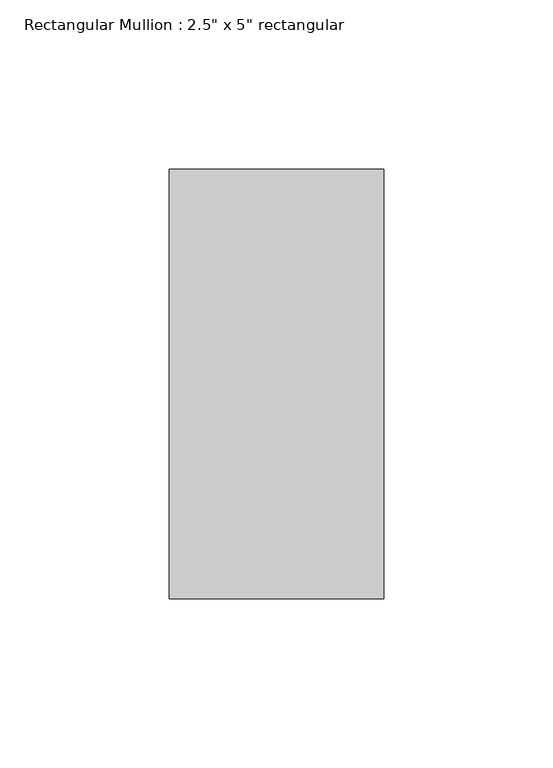
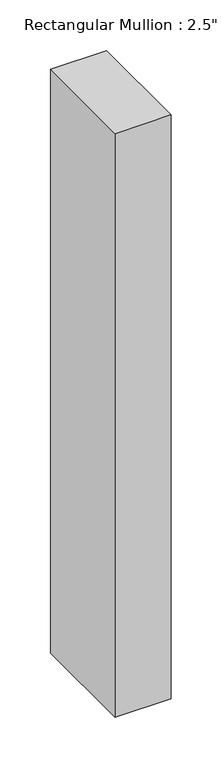
"""IFC4 building model written with IfcOpenShell, lengths in millimetres: member geometry."""

from ifc_helpers import new_model, si_unit, frame, origin, place, context, project, spatial, polyline, outline, extrude, source, transform, mapped, element, save


def member_80b47cb0(model_context):
    return source(origin(), model_context, "Body", "SweptSolid", [
        extrude(outline(polyline([(0.0, 63.5), (0.0, -63.5), (-63.5, -63.5), (-63.5, 63.5), (0.0, 63.5)])), frame((0.0, 0.0, -700.7305927), z_axis=(0.0, 0.0, 1.0), x_axis=(1.0, 0.0, 0.0)), (0.0, 0.0, 1.0), 700.7305927),
    ])


if __name__ == "__main__":
    model = new_model("IFC4")
    model_context = context("Model", 3, world=origin())
    ifc_project = project(units=[si_unit("LENGTHUNIT", "METRE", prefix="MILLI")], contexts=[model_context])
    site = spatial("IfcSite", under=ifc_project)
    building = spatial("IfcBuilding", under=site)
    placement = place(None, origin())
    member_shape = member_80b47cb0(model_context)
    element("IfcMember", 1, ObjectType="Rectangular Mullion : 2.5\" x 5\" rectangular", at=placement, inside=building, context=model_context, shape_type="MappedRepresentation", body=[
        mapped(member_shape, transform((0.0, 0.0, 0.0), x_axis=(1.0, 0.0, 0.0), y_axis=(0.0, 1.0, 0.0), z_axis=(0.0, 0.0, 1.0))),
    ])
    save(model, "model.ifc")

# Revit data of these elements
# Type "Rectangular Mullion : 2.5\" x 5\" rectangular"
#   built-in parameter 1007304 = 0.416667 (stored number, unit not read)
#   built-in parameter 1007301 = 0.104167 (stored number, unit not read)
#   built-in parameter 1007300 = 0.104167 (stored number, unit not read)
# Element 1 (IfcMember, "Rectangular Mullion : 2.5\" x 5\" rectangular")
#   Materials on its faces: "Aluminum"
# Materials
#   "Aluminum": class "Metal", colour RGB 247 247 247, transparency 0, Description = "Aluminum 6061", Cost = 0
